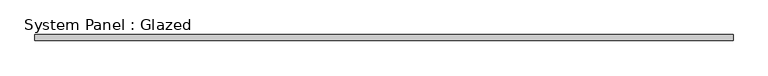
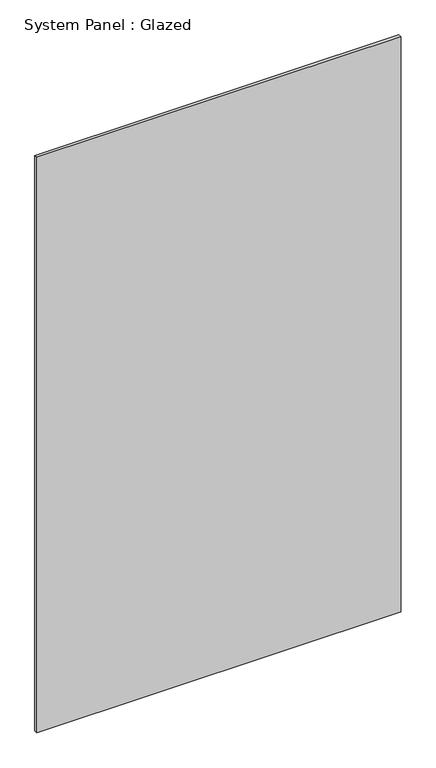
"""IFC4 building model written with IfcOpenShell, lengths in millimetres: plate geometry, System Panel : Glazed."""

from ifc_helpers import new_model, si_unit, origin, origin_with_axes, place, context, project, spatial, polyline, outline, extrude, source, transform, mapped, element, save


def system_panel_glazed_222d0587(model_context):
    return source(origin(), model_context, "Body", "SweptSolid", [
        extrude(outline(polyline([(1460.5, 19.05), (-1460.5, 19.05), (-1460.5, 44.45), (1460.5, 44.45), (1460.5, 19.05)])), origin_with_axes(), (0.0, 0.0, 1.0), 4876.8),
    ])


if __name__ == "__main__":
    model = new_model("IFC4")
    model_context = context("Model", 3, world=origin())
    ifc_project = project(units=[si_unit("LENGTHUNIT", "METRE", prefix="MILLI")], contexts=[model_context])
    site = spatial("IfcSite", under=ifc_project)
    building = spatial("IfcBuilding", under=site)
    placement = place(None, origin())
    system_panel_glazed_shape = system_panel_glazed_222d0587(model_context)
    element("IfcPlate", 1, ObjectType="System Panel : Glazed", at=placement, inside=building, context=model_context, shape_type="MappedRepresentation", body=[
        mapped(system_panel_glazed_shape, transform((0.0, 0.0, 0.0), x_axis=(1.0, 0.0, 0.0), y_axis=(0.0, 1.0, 0.0), z_axis=(0.0, 0.0, 1.0))),
    ])
    save(model, "model.ifc")

# Revit data of these elements
# Type "System Panel : Glazed"
#   Construction Type Id = "GSP4R"
#   Analytic Construction = "1/8 in Pilkington single glazing"
#   Visual Light Transmittance = 0.9
#   Solar Heat Gain Coefficient = 0.86
#   Heat Transfer Coefficient (U) = 1.18115 BTU/(h·ft²·°F)
# Element 1 (IfcPlate, "System Panel : Glazed")
#   Materials on its faces: "Glass"
# Materials
#   "Glass": class "Glass", colour RGB 0 128 192, transparency 0.75, Description = "Soda Lime Glass", Cost = 0
